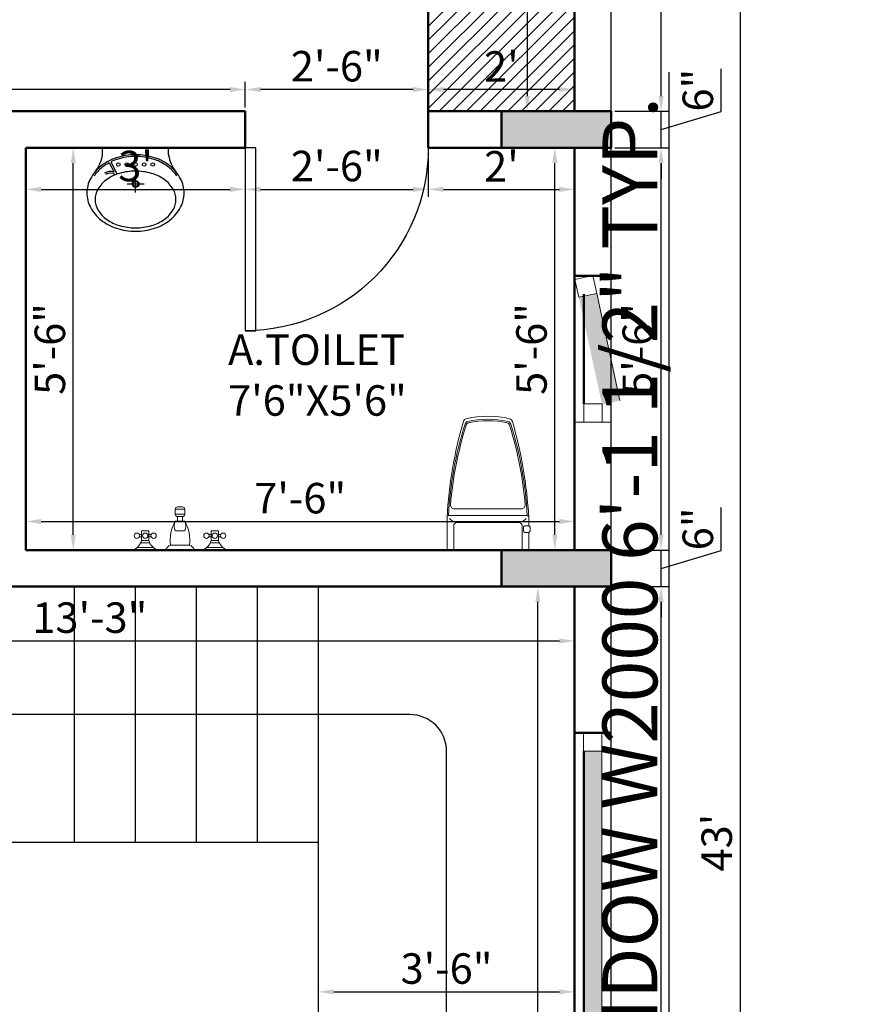
# Model space of a CAD drawing. Units: inches. Extents: x 3064 to 19385, y 846 to 15425.
# Tile 86 of 108: x 7345 to 7482, y 1112 to 1273. Entities that reach past the tile are written whole.
import ezdxf

# ---------------------------------------------------------------- set-up
doc = ezdxf.new("R2010")
doc.units = ezdxf.units.IN
for name, color, linetype, lineweight in [('A-ANNO-DIMS', 2, 'Continuous', 18), ('A-AREA-IDEN', 3, 'Continuous', 18), ('A-COLS', 1, 'Continuous', 35), ('A-DOOR', 3, 'Continuous', 25), ('A-FLOR-FIXT', 9, 'Continuous', 18), ('A-FLOR-STRS', 2, 'Continuous', 25), ('A-FURN-PATT', 252, 'Continuous', 13), ('A-GLAZ', 4, 'Continuous', 18), ('A-WALL', 7, 'Continuous', 50), ('C-PROP', 6, 'Continuous', 25)]:
    doc.layers.add(name, color=color, linetype=linetype, lineweight=lineweight)
doc.layers.add('THIET-BI', color=21, linetype='Continuous')
doc.styles.get("Standard").update_dxf_attribs({"font": 'arial.ttf'})
doc.dimstyles.new('ISO-25', dxfattribs={"dimtxt": 9, "dimasz": 2.5, "dimexe": 1.25, "dimexo": 0.625, "dimtad": 1, "dimdec": 1, "dimlunit": 3, "dimtxsty": 'Standard', "dimcen": 2.5, "dimadec": 0, "dimazin": 0, "dimtfac": 1, "dimtdec": 1, "dimtmove": 0, "dimatfit": 3, "dimfxl": 1, "dimarcsym": 0})

# ---------------------------------------------------------------- blocks, each defined once
blk = doc.blocks.new('*U4')
for p, q in [((0, 0), (0, -6)), ((30, 0), (30, -6))]:
    blk.add_line(p, q)
blk.add_lwpolyline([(0, 0), (0, 30), (1.75, 30), (1.75, 0)], close=True)
blk.add_arc((0, 0), 30, 0, 90)
blk = doc.blocks.new('*D308')
at = {"layer": 'A-ANNO-DIMS', "color": 0, "lineweight": -2, "transparency": 16777216}
for p, q in [((7436.33, 1180.34), (7451.15, 1180.34)), ((7449.9, 984.84), (7449.9, 1177.84)), ((7436.33, 982.34), (7451.15, 982.34))]:
    blk.add_line(p, q, dxfattribs=at)
at = {"layer": 'A-ANNO-DIMS', "color": 0, "transparency": 16777216}
for points in [[(7449.48, 1177.84), (7450.31, 1177.84), (7449.9, 1180.34)], [(7449.48, 984.84), (7450.31, 984.84), (7449.9, 982.34)]]:
    blk.add_solid(points, dxfattribs=at)
at = {"layer": 'Defpoints', "color": 0, "transparency": 16777216}
for p in [(7435.71, 1180.34), (7449.9, 1180.34), (7435.71, 982.34)]:
    blk.add_point(p, dxfattribs=at)
at = {"layer": 'A-ANNO-DIMS', "color": 0, "transparency": 16777216, "insert": (7446.72, 1081.34), "char_height": 5, "attachment_point": 5, "rotation": 90}
blk.add_mtext('16\'-6"', dxfattribs=at)
blk = doc.blocks.new('*D309')
at = {"layer": 'A-ANNO-DIMS', "color": 0, "lineweight": -2, "transparency": 16777216}
for p, q in [((7459.74, 1186.29), (7459.74, 1193.32)), ((7449.9, 1188.84), (7449.9, 1191.34)), ((7442.33, 1186.34), (7451.15, 1186.34)), ((7449.9, 1180.34), (7449.9, 1186.34)), ((7449.9, 1180.34), (7449.9, 1186.34)), ((7449.9, 1183.34), (7459.74, 1186.29)), ((7436.33, 1180.34), (7451.15, 1180.34)), ((7449.9, 1177.84), (7449.9, 1175.34))]:
    blk.add_line(p, q, dxfattribs=at)
at = {"layer": 'A-ANNO-DIMS', "color": 0, "transparency": 16777216}
for points in [[(7449.48, 1188.84), (7450.31, 1188.84), (7449.9, 1186.34)], [(7449.48, 1177.84), (7450.31, 1177.84), (7449.9, 1180.34)]]:
    blk.add_solid(points, dxfattribs=at)
at = {"layer": 'Defpoints', "color": 0, "transparency": 16777216}
for p in [(7441.71, 1186.34), (7449.9, 1186.34), (7435.71, 1180.34)]:
    blk.add_point(p, dxfattribs=at)
at = {"layer": 'A-ANNO-DIMS', "color": 0, "transparency": 16777216, "insert": (7456.57, 1189.81), "char_height": 5, "attachment_point": 5, "rotation": 90}
blk.add_mtext('6"', dxfattribs=at)
blk = doc.blocks.new('*D310')
at = {"layer": 'A-ANNO-DIMS', "color": 0, "lineweight": -2, "transparency": 16777216}
for p, q in [((7442.33, 1252.34), (7451.15, 1252.34)), ((7449.9, 1188.84), (7449.9, 1249.84)), ((7442.33, 1186.34), (7451.15, 1186.34))]:
    blk.add_line(p, q, dxfattribs=at)
at = {"layer": 'A-ANNO-DIMS', "color": 0, "transparency": 16777216}
for points in [[(7449.48, 1249.84), (7450.31, 1249.84), (7449.9, 1252.34)], [(7449.48, 1188.84), (7450.31, 1188.84), (7449.9, 1186.34)]]:
    blk.add_solid(points, dxfattribs=at)
at = {"layer": 'Defpoints', "color": 0, "transparency": 16777216}
for p in [(7441.71, 1252.34), (7449.9, 1252.34), (7441.71, 1186.34)]:
    blk.add_point(p, dxfattribs=at)
at = {"layer": 'A-ANNO-DIMS', "color": 0, "transparency": 16777216, "insert": (7446.72, 1219.34), "char_height": 5, "attachment_point": 5, "rotation": 90}
blk.add_mtext('5\'-6"', dxfattribs=at)
blk = doc.blocks.new('*D311')
at = {"layer": 'A-ANNO-DIMS', "color": 0, "lineweight": -2, "transparency": 16777216}
for p, q in [((7459.74, 1258.29), (7459.74, 1265.32)), ((7449.9, 1260.84), (7449.9, 1263.34)), ((7442.33, 1258.34), (7451.15, 1258.34)), ((7449.9, 1252.34), (7449.9, 1258.34)), ((7449.9, 1252.34), (7449.9, 1258.34)), ((7449.9, 1255.34), (7459.74, 1258.29)), ((7442.33, 1252.34), (7451.15, 1252.34)), ((7449.9, 1249.84), (7449.9, 1247.34))]:
    blk.add_line(p, q, dxfattribs=at)
at = {"layer": 'A-ANNO-DIMS', "color": 0, "transparency": 16777216}
for points in [[(7449.48, 1260.84), (7450.31, 1260.84), (7449.9, 1258.34)], [(7449.48, 1249.84), (7450.31, 1249.84), (7449.9, 1252.34)]]:
    blk.add_solid(points, dxfattribs=at)
at = {"layer": 'Defpoints', "color": 0, "transparency": 16777216}
for p in [(7441.71, 1258.34), (7449.9, 1258.34), (7441.71, 1252.34)]:
    blk.add_point(p, dxfattribs=at)
at = {"layer": 'A-ANNO-DIMS', "color": 0, "transparency": 16777216, "insert": (7456.57, 1261.81), "char_height": 5, "attachment_point": 5, "rotation": 90}
blk.add_mtext('6"', dxfattribs=at)
blk = doc.blocks.new('*D312')
at = {"layer": 'A-ANNO-DIMS', "color": 0, "lineweight": -2, "transparency": 16777216}
for p, q in [((7436.33, 1390.34), (7451.15, 1390.34)), ((7449.9, 1260.84), (7449.9, 1387.84)), ((7442.33, 1258.34), (7451.15, 1258.34))]:
    blk.add_line(p, q, dxfattribs=at)
at = {"layer": 'A-ANNO-DIMS', "color": 0, "transparency": 16777216}
for points in [[(7449.48, 1387.84), (7450.31, 1387.84), (7449.9, 1390.34)], [(7449.48, 1260.84), (7450.31, 1260.84), (7449.9, 1258.34)]]:
    blk.add_solid(points, dxfattribs=at)
at = {"layer": 'Defpoints', "color": 0, "transparency": 16777216}
for p in [(7435.71, 1390.34), (7449.9, 1390.34), (7441.71, 1258.34)]:
    blk.add_point(p, dxfattribs=at)
at = {"layer": 'A-ANNO-DIMS', "color": 0, "transparency": 16777216, "insert": (7446.76, 1324.34), "char_height": 5, "attachment_point": 5, "rotation": 90}
blk.add_mtext("11'", dxfattribs=at)
blk = doc.blocks.new('*D314')
at = {"layer": 'A-ANNO-DIMS', "color": 0, "lineweight": -2, "transparency": 16777216}
for p, q in [((7442.33, 1396.34), (7464.1, 1396.34)), ((7462.85, 1393.84), (7462.85, 882.84)), ((7442.33, 880.34), (7464.1, 880.34))]:
    blk.add_line(p, q, dxfattribs=at)
at = {"layer": 'A-ANNO-DIMS', "color": 0, "transparency": 16777216}
for points in [[(7462.43, 1393.84), (7463.27, 1393.84), (7462.85, 1396.34)], [(7462.43, 882.84), (7463.27, 882.84), (7462.85, 880.34)]]:
    blk.add_solid(points, dxfattribs=at)
at = {"layer": 'Defpoints', "color": 0, "transparency": 16777216}
for p in [(7441.71, 1396.34), (7441.71, 880.34), (7462.85, 880.34)]:
    blk.add_point(p, dxfattribs=at)
at = {"layer": 'A-ANNO-DIMS', "color": 0, "transparency": 16777216, "insert": (7459.67, 1138.34), "char_height": 5, "attachment_point": 5, "rotation": 90}
blk.add_mtext("43'", dxfattribs=at)
blk = doc.blocks.new('*D278')
at = {"layer": 'A-ANNO-DIMS', "color": 0, "lineweight": -2, "transparency": 16777216}
for p, q in [((7435.08, 1390.34), (7426.7, 1390.34)), ((7427.95, 1387.84), (7427.95, 1260.84)), ((7435.08, 1258.34), (7426.7, 1258.34))]:
    blk.add_line(p, q, dxfattribs=at)
at = {"layer": 'A-ANNO-DIMS', "color": 0, "transparency": 16777216}
for points in [[(7427.54, 1387.84), (7428.37, 1387.84), (7427.95, 1390.34)], [(7427.54, 1260.84), (7428.37, 1260.84), (7427.95, 1258.34)]]:
    blk.add_solid(points, dxfattribs=at)
at = {"layer": 'Defpoints', "color": 0, "transparency": 16777216}
for p in [(7435.71, 1390.34), (7427.95, 1258.34), (7435.71, 1258.34)]:
    blk.add_point(p, dxfattribs=at)
at = {"layer": 'A-ANNO-DIMS', "color": 0, "transparency": 16777216, "insert": (7424.82, 1324.34), "char_height": 5, "attachment_point": 5, "rotation": 90}
blk.add_mtext("11'", dxfattribs=at)
blk = doc.blocks.new('*D279')
at = {"layer": 'A-ANNO-DIMS', "color": 0, "lineweight": -2, "transparency": 16777216}
for p, q in [((7411.71, 1258.96), (7411.71, 1263.17)), ((7433.21, 1261.92), (7414.21, 1261.92)), ((7435.71, 1258.96), (7435.71, 1263.17))]:
    blk.add_line(p, q, dxfattribs=at)
at = {"layer": 'A-ANNO-DIMS', "color": 0, "transparency": 16777216}
for points in [[(7414.21, 1262.33), (7414.21, 1261.5), (7411.71, 1261.92)], [(7433.21, 1262.33), (7433.21, 1261.5), (7435.71, 1261.92)]]:
    blk.add_solid(points, dxfattribs=at)
at = {"layer": 'Defpoints', "color": 0, "transparency": 16777216}
for p in [(7411.71, 1261.92), (7411.71, 1258.34), (7435.71, 1258.34)]:
    blk.add_point(p, dxfattribs=at)
at = {"layer": 'A-ANNO-DIMS', "color": 0, "transparency": 16777216, "insert": (7423.71, 1265.05), "char_height": 5, "attachment_point": 5}
blk.add_mtext("2'", dxfattribs=at)
blk = doc.blocks.new('*D280')
at = {"layer": 'A-ANNO-DIMS', "color": 0, "lineweight": -2, "transparency": 16777216}
for p, q in [((7381.71, 1258.96), (7381.71, 1263.17)), ((7409.21, 1261.92), (7384.21, 1261.92)), ((7411.71, 1258.96), (7411.71, 1263.17))]:
    blk.add_line(p, q, dxfattribs=at)
at = {"layer": 'A-ANNO-DIMS', "color": 0, "transparency": 16777216}
for points in [[(7384.21, 1262.33), (7384.21, 1261.5), (7381.71, 1261.92)], [(7409.21, 1262.33), (7409.21, 1261.5), (7411.71, 1261.92)]]:
    blk.add_solid(points, dxfattribs=at)
at = {"layer": 'Defpoints', "color": 0, "transparency": 16777216}
for p in [(7381.71, 1261.92), (7381.71, 1258.34), (7411.71, 1258.34)]:
    blk.add_point(p, dxfattribs=at)
at = {"layer": 'A-ANNO-DIMS', "color": 0, "transparency": 16777216, "insert": (7396.71, 1265.09), "char_height": 5, "attachment_point": 5}
blk.add_mtext('2\'-6"', dxfattribs=at)
blk = doc.blocks.new('*D281')
at = {"layer": 'A-ANNO-DIMS', "color": 0, "lineweight": -2, "transparency": 16777216}
for p, q in [((7276.71, 1258.96), (7276.71, 1263.17)), ((7379.21, 1261.92), (7279.21, 1261.92)), ((7381.71, 1258.96), (7381.71, 1263.17))]:
    blk.add_line(p, q, dxfattribs=at)
at = {"layer": 'A-ANNO-DIMS', "color": 0, "transparency": 16777216}
for points in [[(7279.21, 1262.33), (7279.21, 1261.5), (7276.71, 1261.92)], [(7379.21, 1262.33), (7379.21, 1261.5), (7381.71, 1261.92)]]:
    blk.add_solid(points, dxfattribs=at)
at = {"layer": 'Defpoints', "color": 0, "transparency": 16777216}
for p in [(7276.71, 1261.92), (7276.71, 1258.34), (7381.71, 1258.34)]:
    blk.add_point(p, dxfattribs=at)
at = {"layer": 'A-ANNO-DIMS', "color": 0, "transparency": 16777216, "insert": (7329.21, 1265.09), "char_height": 5, "attachment_point": 5}
blk.add_mtext('8\'-9"', dxfattribs=at)
blk = doc.blocks.new('*D284')
at = {"layer": 'A-ANNO-DIMS', "color": 0, "lineweight": -2, "transparency": 16777216}
for p, q in [((7345.71, 1186.96), (7345.71, 1192.28)), ((7348.21, 1191.03), (7433.21, 1191.03)), ((7435.71, 1186.96), (7435.71, 1192.28))]:
    blk.add_line(p, q, dxfattribs=at)
at = {"layer": 'A-ANNO-DIMS', "color": 0, "transparency": 16777216}
for points in [[(7348.21, 1191.45), (7348.21, 1190.61), (7345.71, 1191.03)], [(7433.21, 1191.45), (7433.21, 1190.61), (7435.71, 1191.03)]]:
    blk.add_solid(points, dxfattribs=at)
at = {"layer": 'Defpoints', "color": 0, "transparency": 16777216}
for p in [(7435.71, 1191.03), (7345.71, 1186.34), (7435.71, 1186.34)]:
    blk.add_point(p, dxfattribs=at)
at = {"layer": 'A-ANNO-DIMS', "color": 0, "transparency": 16777216, "insert": (7390.71, 1194.21), "char_height": 5, "attachment_point": 5}
blk.add_mtext('7\'-6"', dxfattribs=at)
blk = doc.blocks.new('*D285')
at = {"layer": 'A-ANNO-DIMS', "color": 0, "lineweight": -2, "transparency": 16777216}
for p, q in [((7346.33, 1252.34), (7354.73, 1252.34)), ((7353.48, 1188.84), (7353.48, 1249.84)), ((7346.33, 1186.34), (7354.73, 1186.34))]:
    blk.add_line(p, q, dxfattribs=at)
at = {"layer": 'A-ANNO-DIMS', "color": 0, "transparency": 16777216}
for points in [[(7353.07, 1249.84), (7353.9, 1249.84), (7353.48, 1252.34)], [(7353.07, 1188.84), (7353.9, 1188.84), (7353.48, 1186.34)]]:
    blk.add_solid(points, dxfattribs=at)
at = {"layer": 'Defpoints', "color": 0, "transparency": 16777216}
for p in [(7345.71, 1252.34), (7353.48, 1252.34), (7345.71, 1186.34)]:
    blk.add_point(p, dxfattribs=at)
at = {"layer": 'A-ANNO-DIMS', "color": 0, "transparency": 16777216, "insert": (7350.3, 1219.34), "char_height": 5, "attachment_point": 5, "rotation": 90}
blk.add_mtext('5\'-6"', dxfattribs=at)
blk = doc.blocks.new('*D286')
at = {"layer": 'A-ANNO-DIMS', "color": 0, "lineweight": -2, "transparency": 16777216}
for p, q in [((7345.71, 1251.71), (7345.71, 1244.28)), ((7381.71, 1251.71), (7381.71, 1244.28)), ((7348.21, 1245.53), (7379.21, 1245.53))]:
    blk.add_line(p, q, dxfattribs=at)
at = {"layer": 'A-ANNO-DIMS', "color": 0, "transparency": 16777216}
for points in [[(7348.21, 1245.95), (7348.21, 1245.11), (7345.71, 1245.53)], [(7379.21, 1245.95), (7379.21, 1245.11), (7381.71, 1245.53)]]:
    blk.add_solid(points, dxfattribs=at)
at = {"layer": 'Defpoints', "color": 0, "transparency": 16777216}
for p in [(7345.71, 1252.34), (7381.71, 1252.34), (7381.71, 1245.53)]:
    blk.add_point(p, dxfattribs=at)
at = {"layer": 'A-ANNO-DIMS', "color": 0, "transparency": 16777216, "insert": (7363.71, 1248.71), "char_height": 5, "attachment_point": 5}
blk.add_mtext("3'", dxfattribs=at)
blk = doc.blocks.new('*D287')
at = {"layer": 'A-ANNO-DIMS', "color": 0, "lineweight": -2, "transparency": 16777216}
for p, q in [((7381.71, 1251.71), (7381.71, 1244.28)), ((7411.71, 1251.71), (7411.71, 1244.28)), ((7384.21, 1245.53), (7409.21, 1245.53))]:
    blk.add_line(p, q, dxfattribs=at)
at = {"layer": 'A-ANNO-DIMS', "color": 0, "transparency": 16777216}
for points in [[(7384.21, 1245.95), (7384.21, 1245.11), (7381.71, 1245.53)], [(7409.21, 1245.95), (7409.21, 1245.11), (7411.71, 1245.53)]]:
    blk.add_solid(points, dxfattribs=at)
at = {"layer": 'Defpoints', "color": 0, "transparency": 16777216}
for p in [(7381.71, 1252.34), (7411.71, 1252.34), (7411.71, 1245.53)]:
    blk.add_point(p, dxfattribs=at)
at = {"layer": 'A-ANNO-DIMS', "color": 0, "transparency": 16777216, "insert": (7396.71, 1248.71), "char_height": 5, "attachment_point": 5}
blk.add_mtext('2\'-6"', dxfattribs=at)
blk = doc.blocks.new('*D271')
at = {"layer": 'A-ANNO-DIMS', "color": 0, "lineweight": -2, "transparency": 16777216}
for p, q in [((7411.71, 1251.71), (7411.71, 1244.28)), ((7435.71, 1251.71), (7435.71, 1244.28)), ((7414.21, 1245.53), (7433.21, 1245.53))]:
    blk.add_line(p, q, dxfattribs=at)
at = {"layer": 'A-ANNO-DIMS', "color": 0, "transparency": 16777216}
for points in [[(7414.21, 1245.95), (7414.21, 1245.11), (7411.71, 1245.53)], [(7433.21, 1245.95), (7433.21, 1245.11), (7435.71, 1245.53)]]:
    blk.add_solid(points, dxfattribs=at)
at = {"layer": 'Defpoints', "color": 0, "transparency": 16777216}
for p in [(7411.71, 1252.34), (7435.71, 1252.34), (7435.71, 1245.53)]:
    blk.add_point(p, dxfattribs=at)
at = {"layer": 'A-ANNO-DIMS', "color": 0, "transparency": 16777216, "insert": (7423.71, 1248.67), "char_height": 5, "attachment_point": 5}
blk.add_mtext("2'", dxfattribs=at)
blk = doc.blocks.new('*D222')
at = {"layer": 'A-ANNO-DIMS', "color": 0, "lineweight": -2, "transparency": 16777216}
for p, q in [((7435.08, 1252.34), (7431.22, 1252.34)), ((7432.47, 1188.84), (7432.47, 1249.84)), ((7435.08, 1186.34), (7431.22, 1186.34))]:
    blk.add_line(p, q, dxfattribs=at)
at = {"layer": 'A-ANNO-DIMS', "color": 0, "transparency": 16777216}
for points in [[(7432.05, 1249.84), (7432.88, 1249.84), (7432.47, 1252.34)], [(7432.05, 1188.84), (7432.88, 1188.84), (7432.47, 1186.34)]]:
    blk.add_solid(points, dxfattribs=at)
at = {"layer": 'Defpoints', "color": 0, "transparency": 16777216}
for p in [(7432.47, 1252.34), (7435.71, 1252.34), (7435.71, 1186.34)]:
    blk.add_point(p, dxfattribs=at)
at = {"layer": 'A-ANNO-DIMS', "color": 0, "transparency": 16777216, "insert": (7429.29, 1219.34), "char_height": 5, "attachment_point": 5, "rotation": 90}
blk.add_mtext('5\'-6"', dxfattribs=at)
blk = doc.blocks.new('*D237')
at = {"layer": 'A-ANNO-DIMS', "color": 0, "lineweight": -2, "transparency": 16777216}
for p, q in [((7435.08, 1180.34), (7428.45, 1180.34)), ((7429.7, 984.84), (7429.7, 1177.84)), ((7435.08, 982.34), (7428.45, 982.34))]:
    blk.add_line(p, q, dxfattribs=at)
at = {"layer": 'A-ANNO-DIMS', "color": 0, "transparency": 16777216}
for points in [[(7429.28, 1177.84), (7430.12, 1177.84), (7429.7, 1180.34)], [(7429.28, 984.84), (7430.12, 984.84), (7429.7, 982.34)]]:
    blk.add_solid(points, dxfattribs=at)
at = {"layer": 'Defpoints', "color": 0, "transparency": 16777216}
for p in [(7429.7, 1180.34), (7435.71, 1180.34), (7435.71, 982.34)]:
    blk.add_point(p, dxfattribs=at)
at = {"layer": 'A-ANNO-DIMS', "color": 0, "transparency": 16777216, "insert": (7426.52, 1081.34), "char_height": 5, "attachment_point": 5, "rotation": 90}
blk.add_mtext('16\'-6"', dxfattribs=at)
blk = doc.blocks.new('*D238')
at = {"layer": 'A-ANNO-DIMS', "color": 0, "lineweight": -2, "transparency": 16777216}
for p, q in [((7276.71, 1179.71), (7276.71, 1170.17)), ((7435.71, 1179.71), (7435.71, 1170.17)), ((7279.21, 1171.42), (7433.21, 1171.42))]:
    blk.add_line(p, q, dxfattribs=at)
at = {"layer": 'A-ANNO-DIMS', "color": 0, "transparency": 16777216}
for points in [[(7279.21, 1171.84), (7279.21, 1171.01), (7276.71, 1171.42)], [(7433.21, 1171.84), (7433.21, 1171.01), (7435.71, 1171.42)]]:
    blk.add_solid(points, dxfattribs=at)
at = {"layer": 'Defpoints', "color": 0, "transparency": 16777216}
for p in [(7276.71, 1180.34), (7435.71, 1180.34), (7435.71, 1171.42)]:
    blk.add_point(p, dxfattribs=at)
at = {"layer": 'A-ANNO-DIMS', "color": 0, "transparency": 16777216, "insert": (7356.21, 1174.6), "char_height": 5, "attachment_point": 5}
blk.add_mtext('13\'-3"', dxfattribs=at)
blk = doc.blocks.new('*D261')
at = {"layer": 'A-ANNO-DIMS', "color": 0, "lineweight": -2, "transparency": 16777216}
for p, q in [((7393.71, 1114.47), (7393.71, 1115.09)), ((7435.71, 1114.47), (7435.71, 1115.09)), ((7396.21, 1113.84), (7433.21, 1113.84))]:
    blk.add_line(p, q, dxfattribs=at)
at = {"layer": 'A-ANNO-DIMS', "color": 0, "transparency": 16777216}
for points in [[(7396.21, 1114.26), (7396.21, 1113.43), (7393.71, 1113.84)], [(7433.21, 1114.26), (7433.21, 1113.43), (7435.71, 1113.84)]]:
    blk.add_solid(points, dxfattribs=at)
at = {"layer": 'Defpoints', "color": 0, "transparency": 16777216}
for p in [(7393.71, 1113.84), (7435.71, 1113.84), (7435.71, 1113.84)]:
    blk.add_point(p, dxfattribs=at)
at = {"layer": 'A-ANNO-DIMS', "color": 0, "transparency": 16777216, "insert": (7414.71, 1117.02), "char_height": 5, "attachment_point": 5}
blk.add_mtext('3\'-6"', dxfattribs=at)
blk = doc.blocks.new('A$C430D11A0')
at = {"layer": 'THIET-BI'}
for p, q in [((90, 445), (90, 485)), ((475, 485), (90, 485)), ((475, 483), (90, 483)), ((475, 445), (475, 485)), ((138.3, 403), (176, 332.4)), ((129.4, 398.5), (158.2, 344.4)), ((282.5, 226.2), (282.5, 324.8)), ((233.4, 275.5), (331.9, 275.5))]:
    blk.add_line(p, q, dxfattribs=at)
for points in [[(565, 222.5, 0.121635), (544.7, 304.8, 0.10526), (482.3, 379.8, 0.088175), (393.4, 427.4, 0.079002), (282.5, 445, 0.079002), (171.6, 427.4, 0.088175), (82.7, 379.8, 0.10526), (20.3, 304.8, 0.121635), (0, 222.5, 0.121635), (20.3, 140.2, 0.10526), (82.7, 65.2, 0.088175), (171.6, 17.6, 0.079002), (282.5, 0, 0.079002), (393.4, 17.6, 0.088175), (482.3, 65.2, 0.10526), (544.7, 140.2, 0.121635)], [(517.5, 185, 0.134042), (501.2, 244.9, 0.106817), (448.7, 301.7, 0.082468), (375.6, 336.7, 0.070874), (282.5, 350, 0.070874), (189.4, 336.7, 0.082468), (116.3, 301.7, 0.106817), (63.8, 244.9, 0.134042), (47.5, 185, 0.134042), (63.8, 125.1, 0.106817), (116.3, 68.3, 0.082468), (189.4, 33.3, 0.070874), (282.5, 20, 0.070874), (375.6, 33.3, 0.082468), (448.7, 68.3, 0.106817), (501.2, 125.1, 0.134042)]]:
    blk.add_lwpolyline(points, format="xyb", close=True, dxfattribs=at)
for points in [[(522.9, 321.6, 0.07708), (476.1, 372, 0.088175), (390.3, 417.9, 0.079002), (282.5, 435, 0.079002), (174.7, 417.9, 0.035427), (138.3, 403, 0.07708)], [(129.4, 398.5, 0.043566), (88.9, 372, 0.07708), (42.1, 321.6, 0.041486)]]:
    blk.add_lwpolyline(points, format="xyb", dxfattribs=at)
for centre, radius in [((182.5, 388.2), 10.5), ((232.5, 388.2), 10.5), ((282.5, 388.2), 10.5), ((332.5, 388.2), 10.5), ((382.5, 388.2), 10.5), ((282.5, 275.5), 20), ((282.5, 275.5), 15)]:
    blk.add_circle(centre, radius, dxfattribs=at)
for centre, radius, start, end in [((-103.8, 468.9), 195.3, 320.8253, 352.9557), ((668.8, 468.9), 195.3, 187.0443, 219.1747), ((136.4, 285.4), 62.9, 69.643, 123.4774), ((136.4, 285.4), 52.9, 55.2455, 123.4774)]:
    blk.add_arc(centre, radius, start, end, dxfattribs=at)
blk = doc.blocks.new('WC-P05')
for p, q in [((-202.4, 531.6), (-202.4, 439.1)), ((-192.4, 541.6), (262.6, 541.6)), ((-163.4, 541.6), (-163.4, 400.6)), ((233.6, 541.6), (233.6, 400.6)), ((272.6, 531.6), (272.6, 351.6)), ((-210.4, 430.1), (-210.4, 409.1)), ((-201.4, 439.1), (-180.4, 439.1)), ((-171.4, 430.1), (-171.4, 409.1)), ((-202.4, 400.1), (-202.4, 351.6)), ((-201.4, 400.1), (-180.4, 400.1)), ((-166.9, 378.6), (-188.2, 357.3)), ((-143.4, 380.6), (213.6, 380.6)), ((237.1, 378.6), (258.4, 357.3)), ((-192.4, 341.6), (262.6, 341.6)), ((-159.3, 302.6), (229.5, 302.6))]:
    blk.add_line(p, q)
blk.add_lwpolyline([(-90.9, -221.9, 0.114547), (161, -222, 0.114547)], format="xyb")
for centre, radius, start, end in [((-192.4, 531.6), 10, 90, 180), ((262.6, 531.6), 10, 0, 90), ((-201.4, 430.1), 9, 90, 180), ((-201.4, 409.1), 9, 180, 270), ((-180.4, 430.1), 9, 0, 90), ((-180.4, 409.1), 9, 270, 0), ((2308.9, 492.3), 2515.2, 183.2067, 196.1242), ((-192.4, 351.6), 10, 180, 270), ((-143.4, 400.6), 20, 180, 270), ((-2238.7, 492.3), 2515.2, 343.8727, 356.7933), ((213.6, 400.6), 20, 270, 0), ((262.6, 351.6), 10, 270, 0), ((1906, 447.2), 2102.6, 182.8743, 197.6554), ((-159.3, 280.1), 22.5, 90, 184.6246), ((-1835.8, 447.2), 2102.6, 342.3446, 357.1257), ((229.5, 280.1), 22.5, 355.3754, 90), ((1905.9, 447.2), 2094.5, 184.6245, 197.5277), ((-1835.8, 447.2), 2094.6, 342.464, 355.3754), ((-85.8, -199.9), 22.5, 196.1242, 256.8994), ((-76.1, -183.7), 22.5, 197.6554, 257.5059), ((-69.9, -176.8), 22.5, 197.5277, 258.1005), ((35.1, 318), 536.4, 257.5059, 282.4941), ((35.7, 324.3), 534.7, 258.1005, 281.7373), ((139.9, -177.1), 22.5, 281.7373, 342.464), ((146.2, -183.7), 22.5, 282.4941, 342.3446), ((155.9, -200.1), 22.5, 283.0378, 343.8727)]:
    blk.add_arc(centre, radius, start, end)
blk = doc.blocks.new('Faucet - Bathroom front')
for p, q in [((-0.5, 4.25), (0.5, 4.25)), ((0.5, 3.75), (-0.5, 3.75)), ((-0.25, 3), (-0.25, 3.5)), ((0.25, 3.5), (0.25, 3)), ((-0.5, 3), (0.5, 3)), ((-4, 1.625), (-4.25, 1.625)), ((-4, 1.375), (-4.25, 1.375)), ((-3.25, 1.625), (-3, 1.625)), ((-3.25, 1.375), (-3, 1.375)), ((0.5, 2), (-0.5, 2)), ((3.25, 1.625), (3, 1.625)), ((3.25, 1.375), (3, 1.375)), ((4, 1.625), (4.25, 1.625)), ((4, 1.375), (4.25, 1.375)), ((-5, 0), (-2.25, 0)), ((-4.5087, 0.25), (-2.7408, 0.25)), ((-3.1442, 0.75), (-4.0979, 0.75)), ((-1.5, 0), (1.5, 0)), ((-1, 0.5), (1, 0.5)), ((2.25, 0), (5, 0)), ((2.7413, 0.25), (4.5092, 0.25)), ((4.1058, 0.75), (3.1521, 0.75))]:
    blk.add_line(p, q)
for points in [[(-0.5, 3.75), (-0.5, 4.25)], [(-0.25, 4.5), (0.25, 4.5)], [(0.5, 4.25), (0.5, 3.75)], [(0.25, 3.5), (-0.25, 3.5)]]:
    blk.add_lwpolyline(points)
for points in [[(-4, 1), (-4, 2), (-3.25, 2), (-3.25, 1)], [(3.25, 1), (3.25, 2), (4, 2), (4, 1)]]:
    blk.add_lwpolyline(points, close=True)
for centre in [(-4.5, 1.5), (-3.625, 1.5), (-2.75, 1.5), (2.75, 1.5), (3.625, 1.5), (4.5, 1.5)]:
    blk.add_circle(centre, 0.2795)
for centre, radius, start, end in [((-0.2575, 4.2575), 0.2426, 88.22243, 181.7776), ((0.2575, 4.2575), 0.2426, 358.2224, 91.77757), ((-0.2575, 3.7425), 0.2426, 178.2224, 271.7776), ((0.2575, 3.7425), 0.2426, 268.2224, 1.777565), ((3, 1), 4.0311, 150.2551, 187.125), ((0.6413, 2.5), 1.246, 156.3417, 203.6583), ((-3, 1), 4.0311, 352.875, 29.74488), ((-0.6413, 2.5), 1.246, 336.3417, 23.65835), ((-5.375, 1.375), 1.4252, 285.2551, 344.7449), ((-1.875, 1.375), 1.4252, 195.2551, 254.7449), ((-0.7962, -0.2038), 0.7327, 106.1502, 163.8498), ((0.7962, -0.2038), 0.7327, 16.1502, 73.84979), ((1.875, 1.375), 1.4252, 285.2551, 344.7449), ((5.375, 1.375), 1.4252, 195.2551, 254.7449)]:
    blk.add_arc(centre, radius, start, end)
blk = doc.blocks.new('WIN-600')
h = blk.add_hatch(color=256)
h.dxf.hatch_style = 1
h.paths.add_polyline_path([(3, 18), (0, 18), (0, 0), (3, 0)])
blk.add_line((3, 18), (3, 0))
blk.add_lwpolyline([(3, 18), (0, 18), (0, 21), (3, 21)], close=True)
blk = doc.blocks.new('WIN-1800-PAIR')
h = blk.add_hatch(color=256)
h.dxf.hatch_style = 1
h.paths.add_polyline_path([(0, 0), (3, 0), (3, 70.5), (0, 70.5)])
h.paths.add_polyline_path([(3, 144), (0, 144), (0, 73.5), (3, 73.5)])
blk.add_line((3, 144), (3, 73.5))
blk.add_lwpolyline([(3, 144), (0, 144), (0, 147), (3, 147)], close=True)
blk = doc.blocks.new('*D447')
at = {"layer": 'A-ANNO-DIMS', "color": 0, "lineweight": -2, "transparency": 16777216}
for p, q in [((7451.23, 1082.84), (7451.23, 1264.78)), ((7440.83, 1082.84), (7452.48, 1082.84)), ((7451.23, 1011.84), (7451.23, 1080.34)), ((7440.83, 1009.34), (7452.48, 1009.34))]:
    blk.add_line(p, q, dxfattribs=at)
at = {"layer": 'A-ANNO-DIMS', "color": 0, "transparency": 16777216}
for points in [[(7450.81, 1080.34), (7451.65, 1080.34), (7451.23, 1082.84)], [(7450.81, 1011.84), (7451.65, 1011.84), (7451.23, 1009.34)]]:
    blk.add_solid(points, dxfattribs=at)
at = {"layer": 'Defpoints', "color": 0, "transparency": 16777216}
for p in [(7440.21, 1082.84), (7451.23, 1082.84), (7440.21, 1009.34)]:
    blk.add_point(p, dxfattribs=at)
at = {"layer": 'A-ANNO-DIMS', "color": 0, "transparency": 16777216, "insert": (7445.95, 1175.06), "char_height": 9, "attachment_point": 5, "rotation": 90}
blk.add_mtext('WINDOW W2000 6\'-1 1/2" TYP.', dxfattribs=at)

msp = doc.modelspace()

# ---------------------------------------------------------------- hatches: boundary and pattern name
at = {"layer": 'A-COLS'}
h = msp.add_hatch(color=256, dxfattribs=at)
h.dxf.hatch_style = 1
h.paths.add_polyline_path([(7441.71, 1252.34), (7441.71, 1258.34), (7423.71, 1258.34), (7423.71, 1252.34)])
h = msp.add_hatch(color=256, dxfattribs=at)
h.dxf.hatch_style = 1
h.paths.add_polyline_path([(7441.71, 1180.34), (7441.71, 1186.34), (7423.71, 1186.34), (7423.71, 1180.34)])
at = {"layer": 'A-FURN-PATT'}
h = msp.add_hatch(dxfattribs=at)
h.set_pattern_fill('ANSI31', color=256, scale=0.5)
h.set_pattern_definition([(45, (1784.0376, -1e-11), (-1.122532, 1.122532), [])])
h.paths.add_polyline_path([(7411.71, 1258.34), (7435.71, 1258.34), (7435.71, 1390.34), (7411.71, 1390.34)])

# ---------------------------------------------------------------- linework, layer by layer
at = {"layer": 'A-FLOR-STRS'}
for p, q in [((7353.71, 1138.34), (7353.71, 1180.34)), ((7363.71, 1138.34), (7363.71, 1180.34)), ((7373.71, 1138.34), (7373.71, 1180.34)), ((7383.71, 1138.34), (7383.71, 1180.34)), ((7393.71, 1024.34), (7393.71, 1180.34)), ((7393.71, 1138.34), (7293.71, 1138.34))]:
    msp.add_line(p, q, dxfattribs=at)
msp.add_lwpolyline([(7301.19, 1003.34), (7408.71, 1003.34, 0.414214), (7414.71, 1009.34), (7414.71, 1153.34, 0.414214), (7408.71, 1159.34), (7281.71, 1159.34)], format="xyb", dxfattribs=at)
at = {"layer": 'A-GLAZ'}
msp.add_line((7435.71, 1207.34), (7441.71, 1207.34), dxfattribs=at)
msp.add_lwpolyline([(7440.21, 1207.34), (7437.21, 1207.34), (7437.21, 1210.34), (7440.21, 1210.34)], close=True, dxfattribs=at)
at = {"layer": 'A-WALL'}
for p, q in [((7411.71, 1252.34), (7411.71, 1390.34)), ((7435.71, 1258.34), (7435.71, 1390.34)), ((7381.71, 1258.34), (7276.71, 1258.34)), ((7381.71, 1252.34), (7381.71, 1258.34)), ((7411.71, 1252.34), (7411.71, 1258.34)), ((7435.71, 1258.34), (7411.71, 1258.34)), ((7345.71, 1186.34), (7345.71, 1252.34)), ((7381.71, 1252.34), (7345.71, 1252.34)), ((7435.71, 1252.34), (7411.71, 1252.34)), ((7435.71, 1186.34), (7435.71, 1252.34)), ((7435.71, 1231.34), (7441.71, 1231.34)), ((7437.21, 1228.34), (7437.21, 1210.34)), ((7435.71, 1186.34), (7345.71, 1186.34)), ((7435.71, 1180.34), (7276.71, 1180.34)), ((7435.71, 982.34), (7435.71, 1180.34)), ((7441.71, 1156.34), (7435.71, 1156.34)), ((7437.21, 1153.34), (7437.21, 1082.84))]:
    msp.add_line(p, q, dxfattribs=at)
for points in [[(7441.71, 1258.34), (7423.71, 1258.34), (7423.71, 1252.34), (7441.71, 1252.34)], [(7441.71, 1186.34), (7423.71, 1186.34), (7423.71, 1180.34), (7441.71, 1180.34)]]:
    msp.add_lwpolyline(points, close=True, dxfattribs=at)
at = {"layer": 'C-PROP'}
msp.add_line((7441.71, 880.34), (7441.71, 1396.34), dxfattribs=at)

# ---------------------------------------------------------------- block references
at = {"layer": 'A-DOOR', "xscale": -1, "rotation": 180}
msp.add_blockref('*U4', (7381.71, 1252.34), dxfattribs=at)
at = {"layer": 'A-FLOR-FIXT'}
for name, p, xscale, yscale, zscale in [('A$C430D11A0', (7355.73, 1238.65), 0.0282220760332506, 0.0282220760332506, 0.0282220760332506), ('Faucet - Bathroom front', (7371, 1186.34), 1.573166238287219, 1.573166238287219, 1.573166238287219)]:
    msp.add_blockref(name, p, dxfattribs=dict(at, xscale=xscale, yscale=yscale, zscale=zscale))
at = {"layer": 'A-FLOR-FIXT', "xscale": 0.0282220760332506, "yscale": 0.0282220760332506, "zscale": 0.0282220760332506, "rotation": 180}
msp.add_blockref('WC-P05', (7422.48, 1201.63), dxfattribs=at)
at = {"layer": 'A-GLAZ', "rotation": 12.21571913412712}
msp.add_blockref('WIN-600', (7440.21, 1210.23), dxfattribs=at)
at = {"layer": 'A-GLAZ'}
msp.add_blockref('WIN-1800-PAIR', (7437.2, 1009.34), dxfattribs=at)

# ---------------------------------------------------------------- texts
at = {"layer": 'A-AREA-IDEN', "insert": (7378.88, 1221.72), "char_height": 5, "attachment_point": 1}
msp.add_mtext_dynamic_manual_height_columns('A.TOILET\\P7\'6"X5\'6"', width=67.5924, gutter_width=12.5, heights=[0], dxfattribs=at)

# ---------------------------------------------------------------- dimensions: what is measured, and where the dimension line sits
at = {"layer": 'A-ANNO-DIMS'}
for base, p1, p2, override, picture, middle in [((7462.85, 880.34), (7441.71, 1396.34), (7441.71, 880.34), {"dimtxt": 5, "dimclrd": 0, "dimclre": 0, "dimclrt": 0}, '*D314', (7459.67, 1138.34)), ((7427.95, 1258.34), (7435.71, 1390.34), (7435.71, 1258.34), {"dimtxt": 5, "dimclrd": 0, "dimclre": 0, "dimclrt": 0}, '*D278', (7424.82, 1324.34)), ((7449.9, 1390.34), (7441.71, 1258.34), (7435.71, 1390.34), {"dimtxt": 5, "dimclrd": 0, "dimclre": 0, "dimclrt": 0, "dimtmove": 1}, '*D312', (7446.76, 1324.34)), ((7449.9, 1258.34), (7441.71, 1252.34), (7441.71, 1258.34), {"dimtxt": 5, "dimclrd": 0, "dimclre": 0, "dimclrt": 0, "dimtmove": 1}, '*D311', (7456.57, 1258.92)), ((7353.48, 1252.34), (7345.71, 1186.34), (7345.71, 1252.34), {"dimtxt": 5, "dimclrd": 0, "dimclre": 0, "dimclrt": 0}, '*D285', (7350.3, 1219.34)), ((7432.47, 1252.34), (7435.71, 1186.34), (7435.71, 1252.34), {"dimtxt": 5, "dimclrd": 0, "dimclre": 0, "dimclrt": 0}, '*D222', (7429.29, 1219.34)), ((7449.9, 1252.34), (7441.71, 1186.34), (7441.71, 1252.34), {"dimtxt": 5, "dimclrd": 0, "dimclre": 0, "dimclrt": 0, "dimtmove": 1}, '*D310', (7446.72, 1219.34)), ((7449.9, 1186.34), (7435.71, 1180.34), (7441.71, 1186.34), {"dimtxt": 5, "dimclrd": 0, "dimclre": 0, "dimclrt": 0, "dimtmove": 1}, '*D309', (7456.57, 1186.92)), ((7429.7, 1180.34), (7435.71, 982.34), (7435.71, 1180.34), {"dimtxt": 5, "dimclrd": 0, "dimclre": 0, "dimclrt": 0}, '*D237', (7426.52, 1081.34)), ((7449.9, 1180.34), (7435.71, 982.34), (7435.71, 1180.34), {"dimtxt": 5, "dimclrd": 0, "dimclre": 0, "dimclrt": 0, "dimtmove": 1}, '*D308', (7446.72, 1081.34))]:
    dim = msp.add_linear_dim(base=base, p1=p1, p2=p2, angle=90, dimstyle='ISO-25', override=override, dxfattribs=at)
    dim.commit()
    dim.dimension.update_dxf_attribs({"geometry": picture, "text_midpoint": middle})
for base, p1, p2, override, picture, middle in [((7276.71, 1261.92), (7381.71, 1258.34), (7276.71, 1258.34), {"dimtxt": 5, "dimclrd": 0, "dimclre": 0, "dimclrt": 0, "dimtmove": 1}, '*D281', (7329.21, 1265.09)), ((7381.71, 1261.92), (7411.71, 1258.34), (7381.71, 1258.34), {"dimtxt": 5, "dimclrd": 0, "dimclre": 0, "dimclrt": 0, "dimtmove": 1}, '*D280', (7396.71, 1265.09)), ((7411.71, 1261.92), (7435.71, 1258.34), (7411.71, 1258.34), {"dimtxt": 5, "dimclrd": 0, "dimclre": 0, "dimclrt": 0}, '*D279', (7423.71, 1265.05)), ((7381.71, 1245.53), (7345.71, 1252.34), (7381.71, 1252.34), {"dimtxt": 5, "dimclrd": 0, "dimclre": 0, "dimclrt": 0}, '*D286', (7363.71, 1248.71)), ((7411.71, 1245.53), (7381.71, 1252.34), (7411.71, 1252.34), {"dimtxt": 5, "dimclrd": 0, "dimclre": 0, "dimclrt": 0, "dimtmove": 1}, '*D287', (7396.71, 1248.71)), ((7435.71, 1245.53), (7411.71, 1252.34), (7435.71, 1252.34), {"dimtxt": 5, "dimclrd": 0, "dimclre": 0, "dimclrt": 0, "dimtmove": 1}, '*D271', (7423.71, 1248.67)), ((7435.71, 1191.03), (7345.71, 1186.34), (7435.71, 1186.34), {"dimtxt": 5, "dimclrd": 0, "dimclre": 0, "dimclrt": 0}, '*D284', (7390.71, 1194.21)), ((7435.71, 1171.42), (7276.71, 1180.34), (7435.71, 1180.34), {"dimtxt": 5, "dimclrd": 0, "dimclre": 0, "dimclrt": 0}, '*D238', (7356.21, 1174.6)), ((7435.71, 1113.84), (7393.71, 1113.84), (7435.71, 1113.84), {"dimtxt": 5, "dimclrd": 0, "dimclre": 0, "dimclrt": 0}, '*D261', (7414.71, 1117.02))]:
    dim = msp.add_linear_dim(base=base, p1=p1, p2=p2, dimstyle='ISO-25', override=override, dxfattribs=at)
    dim.commit()
    dim.dimension.update_dxf_attribs({"geometry": picture, "text_midpoint": middle})
dim = msp.add_linear_dim(base=(7451.23, 1082.84), p1=(7440.21, 1009.34), p2=(7440.21, 1082.84), angle=90, text='WINDOW W2000 <> TYP.', dimstyle='ISO-25', override={"dimdec": 1, "dimrnd": 0, "dimzin": 1, "dimlunit": 4, "dimfrac": 2}, dxfattribs=at)
dim.commit()
dim.dimension.update_dxf_attribs({"geometry": '*D447', "text_midpoint": (7445.95, 1175.06)})

doc.saveas('drawing.dxf')
